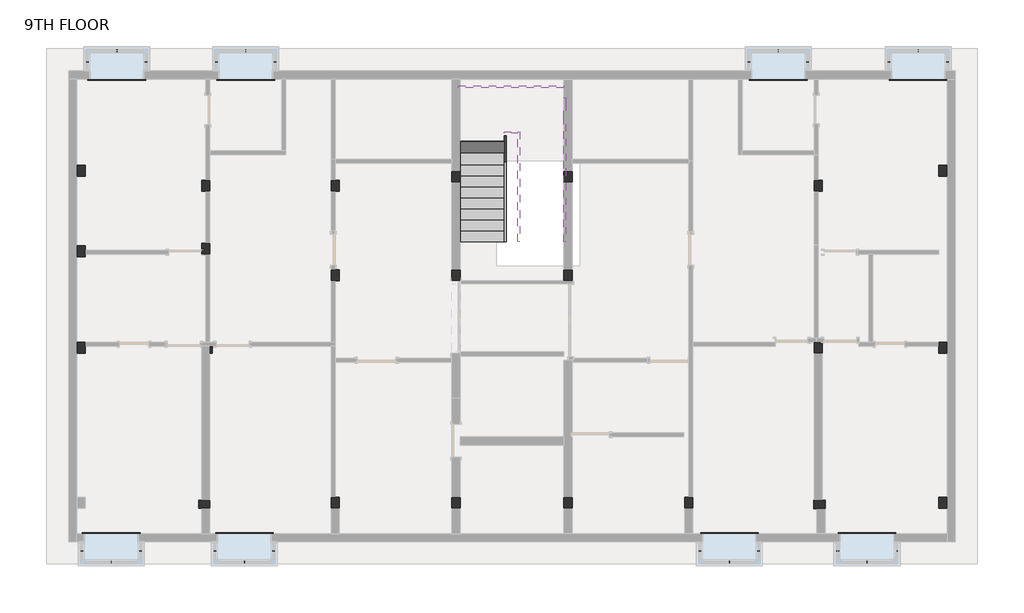
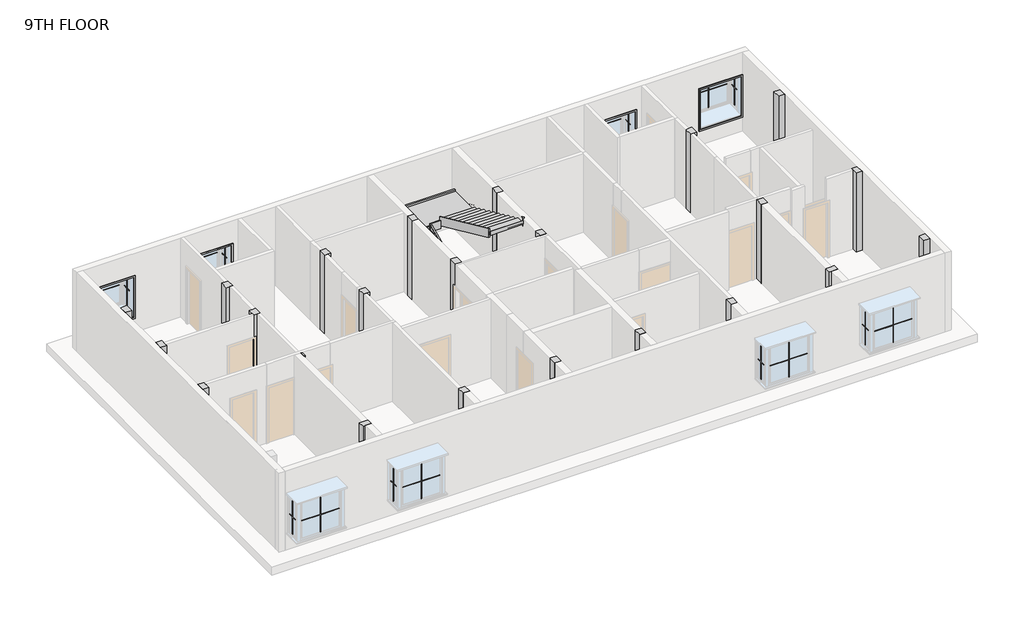
# One storey, part 3 of 3: 32 proxies, 23 columns, 6 members, 1 stair flight.
"""IFC4 building model written with IfcOpenShell, lengths in millimetres."""

from ifc_helpers import new_model, si_unit, frame, origin, place, context, project, spatial, polyline, outline, extrude, faceted_brep, transform, mapped, element, save
from components import m_muntin_pattern_2x2_m_muntin_pattern_2x2_c1fd4460, m_muntin_pattern_2x2_m_muntin_pattern_2x2_777b163a, m_trim_window_interior_flat_picture_frame_44e8afef, stair_flight_8cbe8ac5

model = new_model("IFC4")

# Units and contexts
model_context = context("Model", 3, world=origin())
ifc_project = project(units=[si_unit("LENGTHUNIT", "METRE", prefix="MILLI")], contexts=[model_context])

# Site, building, storey
site = spatial("IfcSite", under=ifc_project)
building = spatial("IfcBuilding", under=site)
storey = spatial("IfcBuildingStorey", under=building, Name="9TH FLOOR", Elevation=32004.0)

# Proxies
placement = place(None, origin())
m_muntin_pattern_2x2_m_muntin_pattern_2x2_shape = m_muntin_pattern_2x2_m_muntin_pattern_2x2_c1fd4460(model_context)
element("IfcBuildingElementProxy", 1, Name="M_Muntin Pattern_2x2 : M_Muntin Pattern_2x2", ObjectType="M_Muntin Pattern_2x2 : M_Muntin Pattern_2x2", at=placement, inside=storey, context=model_context, shape_type="MappedRepresentation", body=[
    mapped(m_muntin_pattern_2x2_m_muntin_pattern_2x2_shape, transform((-11500.7987957, -5499.9182661, 32724.65), x_axis=(-1.0, 0.0, 0.0), y_axis=(0.0, -1.0, 0.0), z_axis=(0.0, 0.0, 1.0))),
])
element("IfcBuildingElementProxy", 2, Name="M_Muntin Pattern_2x2 : M_Muntin Pattern_2x2", ObjectType="M_Muntin Pattern_2x2 : M_Muntin Pattern_2x2", at=placement, inside=storey, context=model_context, shape_type="MappedRepresentation", body=[
    mapped(m_muntin_pattern_2x2_m_muntin_pattern_2x2_shape, transform((-7819.250543, -5499.9182661, 32724.65), x_axis=(-1.0, 0.0, 0.0), y_axis=(0.0, -1.0, 0.0), z_axis=(0.0, 0.0, 1.0))),
])
element("IfcBuildingElementProxy", 3, Name="M_Muntin Pattern_2x2 : M_Muntin Pattern_2x2", ObjectType="M_Muntin Pattern_2x2 : M_Muntin Pattern_2x2", at=placement, inside=storey, context=model_context, shape_type="MappedRepresentation", body=[
    mapped(m_muntin_pattern_2x2_m_muntin_pattern_2x2_shape, transform((5599.7512082, -5499.9182661, 32724.65), x_axis=(-1.0, 0.0, 0.0), y_axis=(0.0, -1.0, 0.0), z_axis=(0.0, 0.0, 1.0))),
])
element("IfcBuildingElementProxy", 4, Name="M_Muntin Pattern_2x2 : M_Muntin Pattern_2x2", ObjectType="M_Muntin Pattern_2x2 : M_Muntin Pattern_2x2", at=placement, inside=storey, context=model_context, shape_type="MappedRepresentation", body=[
    mapped(m_muntin_pattern_2x2_m_muntin_pattern_2x2_shape, transform((9408.6146942, -5499.9182662, 32724.65), x_axis=(-1.0, 0.0, 0.0), y_axis=(0.0, -1.0, 0.0), z_axis=(0.0, 0.0, 1.0))),
])
element("IfcBuildingElementProxy", 5, Name="M_Muntin Pattern_2x2 : M_Muntin Pattern_2x2", ObjectType="M_Muntin Pattern_2x2 : M_Muntin Pattern_2x2", at=placement, inside=storey, context=model_context, shape_type="MappedRepresentation", body=[
    mapped(m_muntin_pattern_2x2_m_muntin_pattern_2x2_shape, transform((-11348.3987957, 8647.7317329, 32724.65), x_axis=(1.0, 0.0, 0.0), y_axis=(0.0, 1.0, 0.0), z_axis=(0.0, 0.0, 1.0))),
])
element("IfcBuildingElementProxy", 6, Name="M_Muntin Pattern_2x2 : M_Muntin Pattern_2x2", ObjectType="M_Muntin Pattern_2x2 : M_Muntin Pattern_2x2", at=placement, inside=storey, context=model_context, shape_type="MappedRepresentation", body=[
    mapped(m_muntin_pattern_2x2_m_muntin_pattern_2x2_shape, transform((-7779.6987993, 8647.7317329, 32724.65), x_axis=(1.0, 0.0, 0.0), y_axis=(0.0, 1.0, 0.0), z_axis=(0.0, 0.0, 1.0))),
])
element("IfcBuildingElementProxy", 7, Name="M_Muntin Pattern_2x2 : M_Muntin Pattern_2x2", ObjectType="M_Muntin Pattern_2x2 : M_Muntin Pattern_2x2", at=placement, inside=storey, context=model_context, shape_type="MappedRepresentation", body=[
    mapped(m_muntin_pattern_2x2_m_muntin_pattern_2x2_shape, transform((6952.301208, 8647.7317329, 32724.65), x_axis=(1.0, 0.0, 0.0), y_axis=(0.0, 1.0, 0.0), z_axis=(0.0, 0.0, 1.0))),
])
element("IfcBuildingElementProxy", 8, Name="M_Muntin Pattern_2x2 : M_Muntin Pattern_2x2", ObjectType="M_Muntin Pattern_2x2 : M_Muntin Pattern_2x2", at=placement, inside=storey, context=model_context, shape_type="MappedRepresentation", body=[
    mapped(m_muntin_pattern_2x2_m_muntin_pattern_2x2_shape, transform((10825.8012075, 8647.7317329, 32724.65), x_axis=(1.0, 0.0, 0.0), y_axis=(0.0, 1.0, 0.0), z_axis=(0.0, 0.0, 1.0))),
])
m_muntin_pattern_2x2_m_muntin_pattern_2x2_2_shape = m_muntin_pattern_2x2_m_muntin_pattern_2x2_777b163a(model_context)
element("IfcBuildingElementProxy", 9, Name="M_Muntin Pattern_2x2 : M_Muntin Pattern_2x2", ObjectType="M_Muntin Pattern_2x2 : M_Muntin Pattern_2x2", at=placement, inside=storey, context=model_context, shape_type="MappedRepresentation", body=[
    mapped(m_muntin_pattern_2x2_m_muntin_pattern_2x2_2_shape, transform((-10690.4737957, -5190.3932661, 32724.65), x_axis=(0.0, 1.0, 0.0), y_axis=(-1.0, 0.0, 0.0), z_axis=(0.0, 0.0, 1.0))),
])
element("IfcBuildingElementProxy", 10, Name="M_Muntin Pattern_2x2 : M_Muntin Pattern_2x2", ObjectType="M_Muntin Pattern_2x2 : M_Muntin Pattern_2x2", at=placement, inside=storey, context=model_context, shape_type="MappedRepresentation", body=[
    mapped(m_muntin_pattern_2x2_m_muntin_pattern_2x2_2_shape, transform((-12311.1237957, -5190.3932661, 32724.65), x_axis=(0.0, -1.0, 0.0), y_axis=(1.0, 0.0, 0.0), z_axis=(0.0, 0.0, 1.0))),
])
element("IfcBuildingElementProxy", 11, Name="M_Muntin Pattern_2x2 : M_Muntin Pattern_2x2", ObjectType="M_Muntin Pattern_2x2 : M_Muntin Pattern_2x2", at=placement, inside=storey, context=model_context, shape_type="MappedRepresentation", body=[
    mapped(m_muntin_pattern_2x2_m_muntin_pattern_2x2_2_shape, transform((-7008.925543, -5190.3932661, 32724.65), x_axis=(0.0, 1.0, 0.0), y_axis=(-1.0, 0.0, 0.0), z_axis=(0.0, 0.0, 1.0))),
])
element("IfcBuildingElementProxy", 12, Name="M_Muntin Pattern_2x2 : M_Muntin Pattern_2x2", ObjectType="M_Muntin Pattern_2x2 : M_Muntin Pattern_2x2", at=placement, inside=storey, context=model_context, shape_type="MappedRepresentation", body=[
    mapped(m_muntin_pattern_2x2_m_muntin_pattern_2x2_2_shape, transform((-8629.575543, -5190.3932661, 32724.65), x_axis=(0.0, -1.0, 0.0), y_axis=(1.0, 0.0, 0.0), z_axis=(0.0, 0.0, 1.0))),
])
element("IfcBuildingElementProxy", 13, Name="M_Muntin Pattern_2x2 : M_Muntin Pattern_2x2", ObjectType="M_Muntin Pattern_2x2 : M_Muntin Pattern_2x2", at=placement, inside=storey, context=model_context, shape_type="MappedRepresentation", body=[
    mapped(m_muntin_pattern_2x2_m_muntin_pattern_2x2_2_shape, transform((6410.0762082, -5190.3932661, 32724.65), x_axis=(0.0, 1.0, 0.0), y_axis=(-1.0, 0.0, 0.0), z_axis=(0.0, 0.0, 1.0))),
])
element("IfcBuildingElementProxy", 14, Name="M_Muntin Pattern_2x2 : M_Muntin Pattern_2x2", ObjectType="M_Muntin Pattern_2x2 : M_Muntin Pattern_2x2", at=placement, inside=storey, context=model_context, shape_type="MappedRepresentation", body=[
    mapped(m_muntin_pattern_2x2_m_muntin_pattern_2x2_2_shape, transform((4789.4262082, -5190.3932661, 32724.65), x_axis=(0.0, -1.0, 0.0), y_axis=(1.0, 0.0, 0.0), z_axis=(0.0, 0.0, 1.0))),
])
element("IfcBuildingElementProxy", 15, Name="M_Muntin Pattern_2x2 : M_Muntin Pattern_2x2", ObjectType="M_Muntin Pattern_2x2 : M_Muntin Pattern_2x2", at=placement, inside=storey, context=model_context, shape_type="MappedRepresentation", body=[
    mapped(m_muntin_pattern_2x2_m_muntin_pattern_2x2_2_shape, transform((10218.9396942, -5190.3932662, 32724.65), x_axis=(0.0, 1.0, 0.0), y_axis=(-1.0, 0.0, 0.0), z_axis=(0.0, 0.0, 1.0))),
])
element("IfcBuildingElementProxy", 16, Name="M_Muntin Pattern_2x2 : M_Muntin Pattern_2x2", ObjectType="M_Muntin Pattern_2x2 : M_Muntin Pattern_2x2", at=placement, inside=storey, context=model_context, shape_type="MappedRepresentation", body=[
    mapped(m_muntin_pattern_2x2_m_muntin_pattern_2x2_2_shape, transform((8598.2896942, -5190.3932661, 32724.65), x_axis=(0.0, -1.0, 0.0), y_axis=(1.0, 0.0, 0.0), z_axis=(0.0, 0.0, 1.0))),
])
element("IfcBuildingElementProxy", 17, Name="M_Muntin Pattern_2x2 : M_Muntin Pattern_2x2", ObjectType="M_Muntin Pattern_2x2 : M_Muntin Pattern_2x2", at=placement, inside=storey, context=model_context, shape_type="MappedRepresentation", body=[
    mapped(m_muntin_pattern_2x2_m_muntin_pattern_2x2_2_shape, transform((-12158.7237957, 8338.2067329, 32724.65), x_axis=(0.0, -1.0, 0.0), y_axis=(1.0, 0.0, 0.0), z_axis=(0.0, 0.0, 1.0))),
])
element("IfcBuildingElementProxy", 18, Name="M_Muntin Pattern_2x2 : M_Muntin Pattern_2x2", ObjectType="M_Muntin Pattern_2x2 : M_Muntin Pattern_2x2", at=placement, inside=storey, context=model_context, shape_type="MappedRepresentation", body=[
    mapped(m_muntin_pattern_2x2_m_muntin_pattern_2x2_2_shape, transform((-10538.0737957, 8338.2067329, 32724.65), x_axis=(0.0, 1.0, 0.0), y_axis=(-1.0, 0.0, 0.0), z_axis=(0.0, 0.0, 1.0))),
])
element("IfcBuildingElementProxy", 19, Name="M_Muntin Pattern_2x2 : M_Muntin Pattern_2x2", ObjectType="M_Muntin Pattern_2x2 : M_Muntin Pattern_2x2", at=placement, inside=storey, context=model_context, shape_type="MappedRepresentation", body=[
    mapped(m_muntin_pattern_2x2_m_muntin_pattern_2x2_2_shape, transform((-8590.0237993, 8338.2067329, 32724.65), x_axis=(0.0, -1.0, 0.0), y_axis=(1.0, 0.0, 0.0), z_axis=(0.0, 0.0, 1.0))),
])
element("IfcBuildingElementProxy", 20, Name="M_Muntin Pattern_2x2 : M_Muntin Pattern_2x2", ObjectType="M_Muntin Pattern_2x2 : M_Muntin Pattern_2x2", at=placement, inside=storey, context=model_context, shape_type="MappedRepresentation", body=[
    mapped(m_muntin_pattern_2x2_m_muntin_pattern_2x2_2_shape, transform((-6969.3737993, 8338.2067329, 32724.65), x_axis=(0.0, 1.0, 0.0), y_axis=(-1.0, 0.0, 0.0), z_axis=(0.0, 0.0, 1.0))),
])
element("IfcBuildingElementProxy", 21, Name="M_Muntin Pattern_2x2 : M_Muntin Pattern_2x2", ObjectType="M_Muntin Pattern_2x2 : M_Muntin Pattern_2x2", at=placement, inside=storey, context=model_context, shape_type="MappedRepresentation", body=[
    mapped(m_muntin_pattern_2x2_m_muntin_pattern_2x2_2_shape, transform((6141.976208, 8338.2067329, 32724.65), x_axis=(0.0, -1.0, 0.0), y_axis=(1.0, 0.0, 0.0), z_axis=(0.0, 0.0, 1.0))),
])
element("IfcBuildingElementProxy", 22, Name="M_Muntin Pattern_2x2 : M_Muntin Pattern_2x2", ObjectType="M_Muntin Pattern_2x2 : M_Muntin Pattern_2x2", at=placement, inside=storey, context=model_context, shape_type="MappedRepresentation", body=[
    mapped(m_muntin_pattern_2x2_m_muntin_pattern_2x2_2_shape, transform((7762.626208, 8338.2067329, 32724.65), x_axis=(0.0, 1.0, 0.0), y_axis=(-1.0, 0.0, 0.0), z_axis=(0.0, 0.0, 1.0))),
])
element("IfcBuildingElementProxy", 23, Name="M_Muntin Pattern_2x2 : M_Muntin Pattern_2x2", ObjectType="M_Muntin Pattern_2x2 : M_Muntin Pattern_2x2", at=placement, inside=storey, context=model_context, shape_type="MappedRepresentation", body=[
    mapped(m_muntin_pattern_2x2_m_muntin_pattern_2x2_2_shape, transform((10015.4762075, 8338.2067329, 32724.65), x_axis=(0.0, -1.0, 0.0), y_axis=(1.0, 0.0, 0.0), z_axis=(0.0, 0.0, 1.0))),
])
element("IfcBuildingElementProxy", 24, Name="M_Muntin Pattern_2x2 : M_Muntin Pattern_2x2", ObjectType="M_Muntin Pattern_2x2 : M_Muntin Pattern_2x2", at=placement, inside=storey, context=model_context, shape_type="MappedRepresentation", body=[
    mapped(m_muntin_pattern_2x2_m_muntin_pattern_2x2_2_shape, transform((11636.1262075, 8338.2067329, 32724.65), x_axis=(0.0, 1.0, 0.0), y_axis=(-1.0, 0.0, 0.0), z_axis=(0.0, 0.0, 1.0))),
])
m_trim_window_interior_flat_picture_frame_shape = m_trim_window_interior_flat_picture_frame_44e8afef(model_context)
element("IfcBuildingElementProxy", 25, Name="M_Trim-Window-Interior-Flat : Picture Frame", ObjectType="M_Trim-Window-Interior-Flat : Picture Frame", at=placement, inside=storey, context=model_context, shape_type="MappedRepresentation", body=[
    mapped(m_trim_window_interior_flat_picture_frame_shape, transform((-11500.7987957, -4712.5932661, 34154.8), x_axis=(-1.0, 0.0, 0.0), y_axis=(0.0, 0.0, 1.0), z_axis=(0.0, 1.0, 0.0))),
])
element("IfcBuildingElementProxy", 26, Name="M_Trim-Window-Interior-Flat : Picture Frame", ObjectType="M_Trim-Window-Interior-Flat : Picture Frame", at=placement, inside=storey, context=model_context, shape_type="MappedRepresentation", body=[
    mapped(m_trim_window_interior_flat_picture_frame_shape, transform((-7819.250543, -4712.5932661, 34154.8), x_axis=(-1.0, 0.0, 0.0), y_axis=(0.0, 0.0, 1.0), z_axis=(0.0, 1.0, 0.0))),
])
element("IfcBuildingElementProxy", 27, Name="M_Trim-Window-Interior-Flat : Picture Frame", ObjectType="M_Trim-Window-Interior-Flat : Picture Frame", at=placement, inside=storey, context=model_context, shape_type="MappedRepresentation", body=[
    mapped(m_trim_window_interior_flat_picture_frame_shape, transform((5599.7512082, -4712.5932661, 34154.8), x_axis=(-1.0, 0.0, 0.0), y_axis=(0.0, 0.0, 1.0), z_axis=(0.0, 1.0, 0.0))),
])
element("IfcBuildingElementProxy", 28, Name="M_Trim-Window-Interior-Flat : Picture Frame", ObjectType="M_Trim-Window-Interior-Flat : Picture Frame", at=placement, inside=storey, context=model_context, shape_type="MappedRepresentation", body=[
    mapped(m_trim_window_interior_flat_picture_frame_shape, transform((9408.6146942, -4712.5932661, 34154.8), x_axis=(-1.0, 0.0, 0.0), y_axis=(0.0, 0.0, 1.0), z_axis=(0.0, 1.0, 0.0))),
])
element("IfcBuildingElementProxy", 29, Name="M_Trim-Window-Interior-Flat : Picture Frame", ObjectType="M_Trim-Window-Interior-Flat : Picture Frame", at=placement, inside=storey, context=model_context, shape_type="MappedRepresentation", body=[
    mapped(m_trim_window_interior_flat_picture_frame_shape, transform((-11348.3987957, 7860.4067329, 34154.8), x_axis=(1.0, 0.0, 0.0), y_axis=(0.0, 0.0, 1.0), z_axis=(0.0, -1.0, 0.0))),
])
element("IfcBuildingElementProxy", 30, Name="M_Trim-Window-Interior-Flat : Picture Frame", ObjectType="M_Trim-Window-Interior-Flat : Picture Frame", at=placement, inside=storey, context=model_context, shape_type="MappedRepresentation", body=[
    mapped(m_trim_window_interior_flat_picture_frame_shape, transform((-7779.6987993, 7860.4067329, 34154.8), x_axis=(1.0, 0.0, 0.0), y_axis=(0.0, 0.0, 1.0), z_axis=(0.0, -1.0, 0.0))),
])
element("IfcBuildingElementProxy", 31, Name="M_Trim-Window-Interior-Flat : Picture Frame", ObjectType="M_Trim-Window-Interior-Flat : Picture Frame", at=placement, inside=storey, context=model_context, shape_type="MappedRepresentation", body=[
    mapped(m_trim_window_interior_flat_picture_frame_shape, transform((6952.301208, 7860.4067329, 34154.8), x_axis=(1.0, 0.0, 0.0), y_axis=(0.0, 0.0, 1.0), z_axis=(0.0, -1.0, 0.0))),
])
element("IfcBuildingElementProxy", 32, Name="M_Trim-Window-Interior-Flat : Picture Frame", ObjectType="M_Trim-Window-Interior-Flat : Picture Frame", at=placement, inside=storey, context=model_context, shape_type="MappedRepresentation", body=[
    mapped(m_trim_window_interior_flat_picture_frame_shape, transform((10825.8012075, 7860.4067329, 34154.8), x_axis=(1.0, 0.0, 0.0), y_axis=(0.0, 0.0, 1.0), z_axis=(0.0, -1.0, 0.0))),
])

# Columns
element("IfcColumn", 33, ObjectType="Rectangular Column : 1'X 9\"", at=placement, inside=storey, context=model_context, shape_type="SweptSolid", body=[
    extrude(outline(polyline([(-12224.6987957, 583.3067334), (-12224.6987957, 278.5067334), (-12453.2987957, 278.5067334), (-12453.2987957, 583.3067334), (-12224.6987957, 583.3067334)])), frame((0.0, 0.0, 32004.0), z_axis=(0.0, 0.0, 1.0), x_axis=(1.0, 0.0, 0.0)), (0.0, 0.0, 1.0), 3048.0),
])
element("IfcColumn", 34, ObjectType="Rectangular Column : 1'X 9\"", at=placement, inside=storey, context=model_context, shape_type="SweptSolid", body=[
    extrude(outline(polyline([(-12224.6987957, 3256.6567332), (-12224.6987957, 2951.8567332), (-12453.2987957, 2951.8567332), (-12453.2987957, 3256.6567332), (-12224.6987957, 3256.6567332)])), frame((0.0, 0.0, 32004.0), z_axis=(0.0, 0.0, 1.0), x_axis=(1.0, 0.0, 0.0)), (0.0, 0.0, 1.0), 3048.0),
])
element("IfcColumn", 35, ObjectType="Rectangular Column : 1'X 9\"", at=placement, inside=storey, context=model_context, shape_type="Brep", body=[
    faceted_brep([(-8770.2987992, 5066.406733, 32004.0), (-8770.2987992, 4761.606733, 32004.0), (-8884.5987992, 4761.606733, 32004.0), (-8998.8987992, 4761.606733, 32004.0), (-8998.8987992, 5066.406733, 32004.0), (-8884.5987992, 5066.406733, 32004.0), (-8770.2987992, 5066.406733, 35052.0), (-8770.2987992, 4761.606733, 35052.0), (-8884.5987992, 4761.606733, 35052.0), (-8998.8987992, 4761.606733, 35052.0), (-8998.8987992, 5066.406733, 35052.0), (-8884.5987992, 5066.406733, 35052.0)], [[[0, 1, 2, 3, 4, 5]], [[6, 7, 1, 0]], [[7, 8, 9, 3, 2, 1]], [[9, 10, 4, 3]], [[10, 11, 6, 0, 5, 4]], [[6, 11, 10, 9, 8, 7]]]),
])
element("IfcColumn", 36, ObjectType="Rectangular Column : 1'X 9\"", at=placement, inside=storey, context=model_context, shape_type="Brep", body=[
    faceted_brep([(-8770.2987992, 3326.5067332, 32004.0), (-8770.2987992, 3021.7067332, 32004.0), (-8884.598796, 3021.7067332, 32004.0), (-8998.8987992, 3021.7067332, 32004.0), (-8998.8987992, 3326.5067332, 32004.0), (-8884.5987992, 3326.5067332, 32004.0), (-8770.2987992, 3326.5067332, 35052.0), (-8770.2987992, 3021.7067332, 35052.0), (-8884.598796, 3021.7067332, 35052.0), (-8998.8987992, 3021.7067332, 35052.0), (-8998.8987992, 3326.5067332, 35052.0), (-8884.5987992, 3326.5067332, 35052.0)], [[[0, 1, 2, 3, 4, 5]], [[6, 7, 1, 0]], [[7, 8, 9, 3, 2, 1]], [[9, 10, 4, 3]], [[10, 11, 6, 0, 5, 4]], [[6, 11, 10, 9, 8, 7]]]),
])
element("IfcColumn", 37, ObjectType="Rectangular Column : 1'X 9\"", at=placement, inside=storey, context=model_context, shape_type="SweptSolid", body=[
    extrude(outline(polyline([(-8713.148796, 278.5067334), (-8771.750543, 278.5067334), (-8771.750543, 469.0067334), (-8713.148796, 469.0067334), (-8713.148796, 278.5067334)])), frame((0.0, 0.0, 32004.0), z_axis=(0.0, 0.0, 1.0), x_axis=(1.0, 0.0, 0.0)), (0.0, 0.0, 1.0), 3048.0),
])
element("IfcColumn", 38, ObjectType="Rectangular Column : 1'X 9\"", at=placement, inside=storey, context=model_context, shape_type="Brep", body=[
    faceted_brep([(-5188.8987995, 5066.406733, 32004.0), (-5188.8987995, 4761.606733, 32004.0), (-5303.1987995, 4761.606733, 32004.0), (-5417.4987995, 4761.606733, 32004.0), (-5417.4987995, 5066.406733, 32004.0), (-5303.1987995, 5066.406733, 32004.0), (-5188.8987995, 5066.406733, 35052.0), (-5188.8987995, 4761.606733, 35052.0), (-5303.1987995, 4761.606733, 35052.0), (-5417.4987995, 4761.606733, 35052.0), (-5417.4987995, 5066.406733, 35052.0), (-5303.1987995, 5066.406733, 35052.0)], [[[0, 1, 2, 3, 4, 5]], [[6, 7, 1, 0]], [[7, 8, 9, 3, 2, 1]], [[9, 10, 4, 3]], [[10, 11, 6, 0, 5, 4]], [[6, 11, 10, 9, 8, 7]]]),
])
element("IfcColumn", 39, ObjectType="Rectangular Column : 1'X 9\"", at=placement, inside=storey, context=model_context, shape_type="Brep", body=[
    faceted_brep([(-5188.8987995, 2589.9067802, 32004.0), (-5188.8987995, 2285.1067802, 32004.0), (-5303.1987995, 2285.1067802, 32004.0), (-5417.4987995, 2285.1067802, 32004.0), (-5417.4987995, 2589.9067802, 32004.0), (-5303.1987995, 2589.9067802, 32004.0), (-5188.8987995, 2589.9067802, 35052.0), (-5188.8987995, 2285.1067802, 35052.0), (-5303.1987995, 2285.1067802, 35052.0), (-5417.4987995, 2285.1067802, 35052.0), (-5417.4987995, 2589.9067802, 35052.0), (-5303.1987995, 2589.9067802, 35052.0)], [[[0, 1, 2, 3, 4, 5]], [[6, 7, 1, 0]], [[7, 8, 9, 3, 2, 1]], [[9, 10, 4, 3]], [[10, 11, 6, 0, 5, 4]], [[6, 11, 10, 9, 8, 7]]]),
])
element("IfcColumn", 40, ObjectType="Rectangular Column : 1'X 9\"", at=placement, inside=storey, context=model_context, shape_type="Brep", body=[
    faceted_brep([(-5188.8987963, -3709.2932193, 32004.0), (-5188.8987963, -4014.0932193, 32004.0), (-5417.4987963, -4014.0932193, 32004.0), (-5417.4987963, -3709.2932193, 32004.0), (-5303.1987995, -3709.2932193, 32004.0), (-5188.8987963, -3709.2932193, 35052.0), (-5188.8987963, -4014.0932193, 35052.0), (-5417.4987963, -4014.0932193, 35052.0), (-5417.4987963, -3709.2932193, 35052.0), (-5303.1987995, -3709.2932193, 35052.0)], [[[0, 1, 2, 3, 4]], [[5, 6, 1, 0]], [[6, 7, 2, 1]], [[7, 8, 3, 2]], [[8, 9, 5, 0, 4, 3]], [[5, 9, 8, 7, 6]]]),
])
element("IfcColumn", 41, ObjectType="Rectangular Column : 1'X 9\"", at=placement, inside=storey, context=model_context, shape_type="SweptSolid", body=[
    extrude(outline(polyline([(1250.0012085, -3709.2932193), (1250.0012085, -4014.0932193), (1021.4012085, -4014.0932193), (1021.4012085, -3709.2932193), (1250.0012085, -3709.2932193)])), frame((0.0, 0.0, 32004.0), z_axis=(0.0, 0.0, 1.0), x_axis=(1.0, 0.0, 0.0)), (0.0, 0.0, 1.0), 3048.0),
])
element("IfcColumn", 42, ObjectType="Rectangular Column : 1'X 9\"", at=placement, inside=storey, context=model_context, shape_type="Brep", body=[
    faceted_brep([(4590.1012082, -3709.2932193, 32004.0), (4590.1012082, -4014.0932193, 32004.0), (4361.5012082, -4014.0932193, 32004.0), (4361.5012082, -3709.2932193, 32004.0), (4475.8012082, -3709.2932193, 32004.0), (4590.1012082, -3709.2932193, 35052.0), (4590.1012082, -4014.0932193, 35052.0), (4361.5012082, -4014.0932193, 35052.0), (4361.5012082, -3709.2932193, 35052.0), (4475.8012082, -3709.2932193, 35052.0)], [[[0, 1, 2, 3, 4]], [[5, 6, 1, 0]], [[6, 7, 2, 1]], [[7, 8, 3, 2]], [[8, 9, 5, 0, 4, 3]], [[5, 9, 8, 7, 6]]]),
])
element("IfcColumn", 43, ObjectType="Rectangular Column : 1'X 9\"", at=placement, inside=storey, context=model_context, shape_type="SweptSolid", body=[
    extrude(outline(polyline([(11625.9012075, -3709.2932671), (11625.9012075, -4014.0932671), (11397.3012075, -4014.0932671), (11397.3012075, -3709.2932671), (11625.9012075, -3709.2932671)])), frame((0.0, 0.0, 32004.0), z_axis=(0.0, 0.0, 1.0), x_axis=(1.0, 0.0, 0.0)), (0.0, 0.0, 1.0), 3048.0),
])
element("IfcColumn", 44, ObjectType="Rectangular Column : 1'X 9\"", at=placement, inside=storey, context=model_context, shape_type="Brep", body=[
    faceted_brep([(11625.9012075, 583.3067295, 32004.0), (11625.9012075, 278.5067295, 32004.0), (11397.3012075, 278.5067295, 32004.0), (11397.3012075, 469.0067295, 32004.0), (11397.3012075, 583.3067295, 32004.0), (11625.9012075, 583.3067295, 35052.0), (11625.9012075, 278.5067295, 35052.0), (11397.3012075, 278.5067295, 35052.0), (11397.3012075, 469.0067295, 35052.0), (11397.3012075, 583.3067295, 35052.0)], [[[0, 1, 2, 3, 4]], [[5, 6, 1, 0]], [[6, 7, 2, 1]], [[7, 8, 9, 4, 3, 2]], [[9, 5, 0, 4]], [[5, 9, 8, 7, 6]]]),
])
element("IfcColumn", 45, ObjectType="Rectangular Column : 1'X 9\"", at=placement, inside=storey, context=model_context, shape_type="SweptSolid", body=[
    extrude(outline(polyline([(11625.9012075, 5479.1567329), (11625.9012075, 5174.3567329), (11397.3012075, 5174.3567329), (11397.3012075, 5479.1567329), (11625.9012075, 5479.1567329)])), frame((0.0, 0.0, 32004.0), z_axis=(0.0, 0.0, 1.0), x_axis=(1.0, 0.0, 0.0)), (0.0, 0.0, 1.0), 3048.0),
])
element("IfcColumn", 46, ObjectType="Rectangular Column : 1'X 9\"", at=placement, inside=storey, context=model_context, shape_type="Brep", body=[
    faceted_brep([(8172.5040565, 5065.4824989, 32004.0), (8172.5040565, 4760.6824989, 32004.0), (8057.2012047, 4760.6824989, 32004.0), (7943.9040565, 4760.6824989, 32004.0), (7943.9040565, 5065.4824989, 32004.0), (8058.2040565, 5065.4824989, 32004.0), (8172.5040565, 5065.4824989, 35052.0), (8172.5040565, 4760.6824989, 35052.0), (8057.2012047, 4760.6824989, 35052.0), (7943.9040565, 4760.6824989, 35052.0), (7943.9040565, 5065.4824989, 35052.0), (8058.2040565, 5065.4824989, 35052.0)], [[[0, 1, 2, 3, 4, 5]], [[6, 7, 1, 0]], [[7, 8, 9, 3, 2, 1]], [[9, 10, 4, 3]], [[10, 11, 6, 0, 5, 4]], [[6, 11, 10, 9, 8, 7]]]),
])
element("IfcColumn", 47, ObjectType="Rectangular Column : 1'X 9\"", at=placement, inside=storey, context=model_context, shape_type="Brep", body=[
    faceted_brep([(8171.5012047, 583.3067334, 32004.0), (8171.5012047, 278.5067334, 32004.0), (7942.9012047, 278.5067334, 32004.0), (7942.9012047, 583.3067334, 32004.0), (8000.0512079, 583.3067334, 32004.0), (8171.5012047, 583.3067334, 35052.0), (8171.5012047, 278.5067334, 35052.0), (7942.9012047, 278.5067334, 35052.0), (7942.9012047, 583.3067334, 35052.0), (8000.0512079, 583.3067334, 35052.0)], [[[0, 1, 2, 3, 4]], [[5, 6, 1, 0]], [[6, 7, 2, 1]], [[7, 8, 3, 2]], [[8, 9, 5, 0, 4, 3]], [[5, 9, 8, 7, 6]]]),
])
element("IfcColumn", 48, ObjectType="Rectangular Column : 1'X 9\"", at=placement, inside=storey, context=model_context, shape_type="Brep", body=[
    faceted_brep([(-9076.550543, -3785.4932196, 32004.0), (-9000.350543, -3785.4932196, 32004.0), (-8771.750543, -3785.4932196, 32004.0), (-8771.750543, -4014.0932196, 32004.0), (-9000.350543, -4014.0932196, 32004.0), (-9076.550543, -4014.0932196, 32004.0), (-9076.550543, -3785.4932196, 35052.0), (-9000.350543, -3785.4932196, 35052.0), (-8771.750543, -3785.4932196, 35052.0), (-8771.750543, -4014.0932196, 35052.0), (-9000.350543, -4014.0932196, 35052.0), (-9076.550543, -4014.0932196, 35052.0)], [[[0, 1, 2, 3, 4, 5]], [[6, 7, 8, 2, 1, 0]], [[8, 9, 3, 2]], [[9, 10, 11, 5, 4, 3]], [[11, 6, 0, 5]], [[6, 11, 10, 9, 8, 7]]]),
])
element("IfcColumn", 49, ObjectType="Rectangular Column : 1'X 9\"", at=placement, inside=storey, context=model_context, shape_type="Brep", body=[
    faceted_brep([(7941.7646942, -3787.3914801, 32004.0), (8246.5646942, -3787.3914801, 32004.0), (8246.5646942, -4015.9914801, 32004.0), (8017.9646942, -4015.9914801, 32004.0), (7941.7646942, -4015.9914801, 32004.0), (7941.7646942, -3787.3914801, 35052.0), (8246.5646942, -3787.3914801, 35052.0), (8246.5646942, -4015.9914801, 35052.0), (8017.9646942, -4015.9914801, 35052.0), (7941.7646942, -4015.9914801, 35052.0)], [[[0, 1, 2, 3, 4]], [[5, 6, 1, 0]], [[6, 7, 2, 1]], [[7, 8, 9, 4, 3, 2]], [[9, 5, 0, 4]], [[5, 9, 8, 7, 6]]]),
])
element("IfcColumn", 50, ObjectType="Rectangular Column : 1'X 9\"", at=placement, inside=storey, context=model_context, shape_type="SweptSolid", body=[
    extrude(outline(polyline([(-12453.2987957, 5174.3567339), (-12453.2987957, 5479.1567339), (-12224.6987957, 5479.1567339), (-12224.6987957, 5174.3567339), (-12453.2987957, 5174.3567339)])), frame((0.0, 0.0, 32004.0), z_axis=(0.0, 0.0, 1.0), x_axis=(1.0, 0.0, 0.0)), (0.0, 0.0, 1.0), 3048.0),
])
element("IfcColumn", 51, ObjectType="Rectangular Column : 1'X 9\"", at=placement, inside=storey, context=model_context, shape_type="SweptSolid", body=[
    extrude(outline(polyline([(-1845.5417538, 5320.4067329), (-1845.5417538, 5015.6067329), (-2074.1417538, 5015.6067329), (-2074.1417538, 5320.4067329), (-1845.5417538, 5320.4067329)])), frame((0.0, 0.0, 32004.0), z_axis=(0.0, 0.0, 1.0), x_axis=(1.0, 0.0, 0.0)), (0.0, 0.0, 1.0), 3048.0),
])
element("IfcColumn", 52, ObjectType="Rectangular Column : 1'X 9\"", at=placement, inside=storey, context=model_context, shape_type="SweptSolid", body=[
    extrude(outline(polyline([(1250.0012085, 5320.4067329), (1250.0012085, 5015.6067329), (1021.4012085, 5015.6067329), (1021.4012085, 5320.4067329), (1250.0012085, 5320.4067329)])), frame((0.0, 0.0, 32004.0), z_axis=(0.0, 0.0, 1.0), x_axis=(1.0, 0.0, 0.0)), (0.0, 0.0, 1.0), 3048.0),
])
element("IfcColumn", 53, ObjectType="Rectangular Column : 1'X 9\"", at=placement, inside=storey, context=model_context, shape_type="SweptSolid", body=[
    extrude(outline(polyline([(-1845.5417538, 2589.906774), (-1845.5417538, 2285.106774), (-2074.1417538, 2285.106774), (-2074.1417538, 2589.906774), (-1845.5417538, 2589.906774)])), frame((0.0, 0.0, 32004.0), z_axis=(0.0, 0.0, 1.0), x_axis=(1.0, 0.0, 0.0)), (0.0, 0.0, 1.0), 3048.0),
])
element("IfcColumn", 54, ObjectType="Rectangular Column : 1'X 9\"", at=placement, inside=storey, context=model_context, shape_type="Brep", body=[
    faceted_brep([(1253.2582462, 2589.9067742, 32004.0), (1253.2582462, 2285.1067742, 32004.0), (1024.6582462, 2285.1067742, 32004.0), (1024.6582462, 2589.9067742, 32004.0), (1250.0012085, 2589.9067742, 32004.0), (1253.2582462, 2589.9067742, 35052.0), (1253.2582462, 2285.1067742, 35052.0), (1024.6582462, 2285.1067742, 35052.0), (1024.6582462, 2589.9067742, 35052.0), (1250.0012085, 2589.9067742, 35052.0)], [[[0, 1, 2, 3, 4]], [[5, 6, 1, 0]], [[6, 7, 2, 1]], [[7, 8, 3, 2]], [[8, 9, 5, 0, 4, 3]], [[5, 9, 8, 7, 6]]]),
])
element("IfcColumn", 55, ObjectType="Rectangular Column : 1'X 9\"", at=placement, inside=storey, context=model_context, shape_type="SweptSolid", body=[
    extrude(outline(polyline([(-1848.7987998, -3709.2932663), (-1848.7987998, -4014.0932663), (-2077.3987998, -4014.0932663), (-2077.3987998, -3709.2932663), (-1848.7987998, -3709.2932663)])), frame((0.0, 0.0, 32004.0), z_axis=(0.0, 0.0, 1.0), x_axis=(1.0, 0.0, 0.0)), (0.0, 0.0, 1.0), 3048.0),
])

# Members
element("IfcMember", 56, ObjectType="Stringer - 2\" Width", at=placement, inside=storey, context=model_context, shape_type="SweptSolid", body=[
    extrude(outline(polyline([(3364.6067329, 32004.0), (3364.6067329, 32203.8262721), (6445.4289342, 33604.2), (7182.0114168, 33604.2), (3661.5714168, 32004.0), (3364.6067329, 32004.0)])), frame((-1896.3417538, 0.0, 0.0), z_axis=(1.0, 0.0, 0.0), x_axis=(0.0, 1.0, 0.0)), (0.0, 0.0, 1.0), 50.8),
])
element("IfcMember", 57, ObjectType="Stringer - 2\" Width", at=placement, inside=storey, context=model_context, shape_type="SweptSolid", body=[
    extrude(outline(polyline([(-1896.3417538, 7631.8067329), (-1896.3417538, 7682.6067329), (1021.4012085, 7682.6067329), (1021.4012085, 7631.8067329), (-1896.3417538, 7631.8067329)])), frame((0.0, 0.0, 33299.4), z_axis=(0.0, 0.0, 1.0), x_axis=(1.0, 0.0, 0.0)), (0.0, 0.0, 1.0), 304.8),
])
element("IfcMember", 58, ObjectType="Stringer - 2\" Width", at=placement, inside=storey, context=model_context, shape_type="SweptSolid", body=[
    extrude(outline(polyline([(6618.562049, 33299.4), (3364.6067329, 34778.4705982), (3364.6067329, 35113.2808176), (7355.1445316, 33299.4), (6618.562049, 33299.4)])), frame((1021.4012085, 0.0, 0.0), z_axis=(1.0, 0.0, 0.0), x_axis=(0.0, 1.0, 0.0)), (0.0, 0.0, 1.0), 50.8),
])
element("IfcMember", 59, ObjectType="Stringer - 2\" Width", at=placement, inside=storey, context=model_context, shape_type="SweptSolid", body=[
    extrude(outline(polyline([(3364.6067329, 32004.0), (3364.6067329, 32203.8262721), (6361.8067329, 33566.1899085), (6361.8067329, 33231.3796892), (3661.5714168, 32004.0), (3364.6067329, 32004.0)])), frame((-629.5987998, 0.0, 0.0), z_axis=(1.0, 0.0, 0.0), x_axis=(0.0, 1.0, 0.0)), (0.0, 0.0, 1.0), 50.8),
])
element("IfcMember", 60, ObjectType="Stringer - 2\" Width", at=placement, inside=storey, context=model_context, shape_type="SweptSolid", body=[
    extrude(outline(polyline([(-629.5987998, 6361.8067329), (-629.5987998, 6412.6067329), (-248.5987915, 6412.6067329), (-248.5987915, 6361.8067329), (-629.5987998, 6361.8067329)])), frame((0.0, 0.0, 33299.4), z_axis=(0.0, 0.0, 1.0), x_axis=(1.0, 0.0, 0.0)), (0.0, 0.0, 1.0), 304.8),
])
element("IfcMember", 61, ObjectType="Stringer - 2\" Width", at=placement, inside=storey, context=model_context, shape_type="SweptSolid", body=[
    extrude(outline(polyline([(6412.6067329, 33727.8262721), (6412.6067329, 33393.0160528), (3364.6067329, 34778.4705982), (3364.6067329, 35113.2808176), (6412.6067329, 33727.8262721)])), frame((-248.5987915, 0.0, 0.0), z_axis=(1.0, 0.0, 0.0), x_axis=(0.0, 1.0, 0.0)), (0.0, 0.0, 1.0), 50.8),
])

# Stair flight
stair_flight_shape = stair_flight_8cbe8ac5(model_context)
element("IfcStairFlight", 62, ObjectType="2\" Tread 1\" Nosing 1/4\" Riser", at=placement, inside=storey, context=model_context, shape_type="MappedRepresentation", body=[
    mapped(stair_flight_shape, transform((0.0, 0.0, 0.0), x_axis=(1.0, 0.0, 0.0), y_axis=(0.0, 1.0, 0.0), z_axis=(0.0, 0.0, 1.0))),
])

save(model, "model.ifc")

# Revit data of these elements
# Type "M_Muntin Pattern_2x2 : M_Muntin Pattern_2x2"
#   Width [instance default] = 3' - 11.24409"
#   Thickness = 0' - 0 1/2"
#   Height [instance default] = 3' - 11.24409"
#   Distance = 0' - 0 3/4"
#   Interior Material [instance default] = none
#   Exterior Material [instance default] = none
#   Default Elevation = 0
# Type "M_Trim-Window-Interior-Flat : Picture Frame"
#   Trim Thickness_Picture Frame = 0' - 1.1811"
#   Trim Width = 0' - 2.3622"
#   Trim Thickness_with Sill = 0' - 0.7874"
#   Sill Thickness = 0' - 1.1811"
#   Opening Width [instance default] = 1' - 11.62205"
#   Opening Height [instance default] = 2' - 11.43307"
#   Default Elevation = 3' - 11.24409"
#   Sill = no
#   Picture Frame = yes
#   Trim Material [instance default] = none
# Type "Rectangular Column : 1'X 9\""
#   Assembly Code = "B1010200"
#   Depth = 1' - 0"
#   Offset Base = 0' - 0"
#   Offset Top = 0' - 0"
#   Width = 0' - 9"
#   Material = none
# Elements 1, 2, 3, 4, 5, 6, 7, 8 (IfcBuildingElementProxy, "M_Muntin Pattern_2x2 : M_Muntin Pattern_2x2")
#   Width = 4' - 5.55512"
#   Height = 4' - 5.55512"
#   Interior Material = Wood - Stained
#   Exterior Material = Clad - White
#   Phase Created = New Construction
#   Materials on its faces: "Clad - White", "Wood - Stained"
# Elements 9, 10, 11, 12, 13, 14, 15, 16, 17, 18, 19, 20, 21, 22, 23, 24 (IfcBuildingElementProxy, "M_Muntin Pattern_2x2 : M_Muntin Pattern_2x2")
#   Width = 1' - 2.12205"
#   Height = 4' - 5.55512"
#   Interior Material = Wood - Stained
#   Exterior Material = Clad - White
#   Phase Created = New Construction
#   Materials on its faces: "Clad - White", "Wood - Stained"
# Elements 25, 26, 27, 28, 29, 30, 31, 32 (IfcBuildingElementProxy, "M_Trim-Window-Interior-Flat : Picture Frame")
#   Opening Width = 4' - 11.05512"
#   Opening Height = 5' - 1.05512"
#   Trim Material = Wood - Stained
#   Phase Created = New Construction
#   Materials on its faces: "Wood - Stained"
# Elements 33, 34, 35, 36, 37, 38, 39, 40, 41, 42, 43, 44, 45, 46, 47, 48, 49, 50, 51, 52, 53, 54, 55 (IfcColumn, "Rectangular Column : 1'X 9\"")
#   Phase Created = New Construction
#   Materials on its faces: "Default Wall"
# Elements 56, 57, 58, 59, 60, 61 (IfcMember, "Stringer - 2\" Width")
#   Phase Created = New Construction
# Element 62 (IfcStairFlight, "2\" Tread 1\" Nosing 1/4\" Riser")
#   Phase Created = New Construction
# Materials
#   "Clad - White": class "Wood", colour RGB 242 242 238, transparency 0, Cost = 0
#   "Wood - Stained": class "Wood", colour RGB 224 178 126, transparency 0, Cost = 0
#   "Default Wall": colour RGB 128 128 128, transparency 0, Cost = 0
